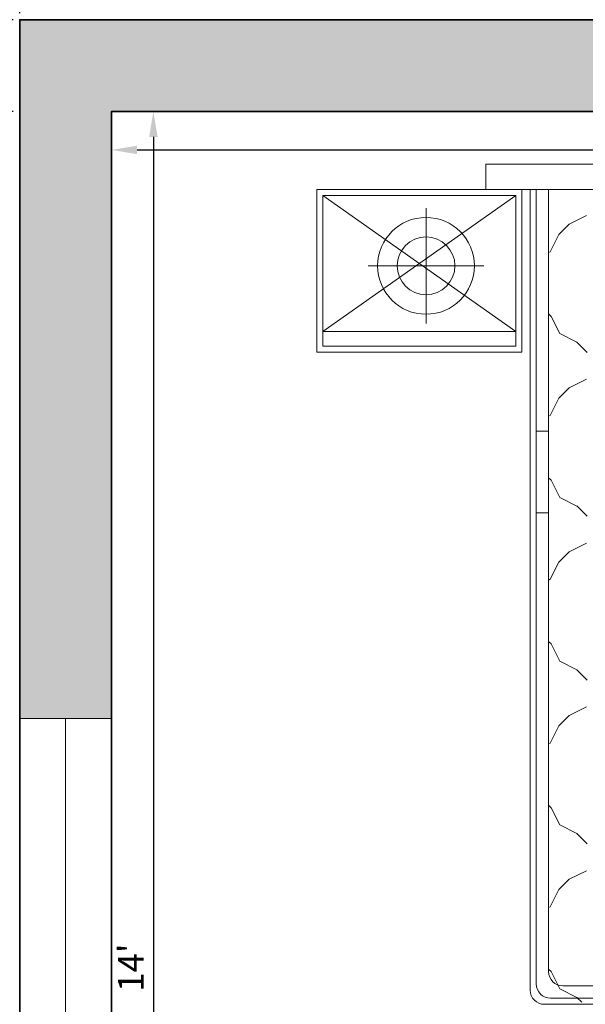
# Model space of a CAD drawing. Units: inches. Extents: x 2901 to 5923, y 918 to 2827.
# Tile 5 of 16: x 4430 to 4486, y 1534 to 1630. Entities that reach past the tile are written whole.
import ezdxf

# ---------------------------------------------------------------- set-up
doc = ezdxf.new("R2010")
doc.units = ezdxf.units.IN
for name, color, linetype, lineweight in [('A-ANNO-DIMS', 2, 'Continuous', 18), ('A-GLAZ', 4, 'Continuous', 18), ('A-WALL-PATT', 7, 'Continuous', 13), ('furniture', 160, 'Continuous', 18), ('walls', 7, 'Continuous', 35)]:
    doc.layers.add(name, color=color, linetype=linetype, lineweight=lineweight)
doc.styles.get("Standard").update_dxf_attribs({"font": 'arial.ttf'})
doc.dimstyles.new('Copy of ISO-25', dxfattribs={"dimtxt": 2.5, "dimasz": 2.5, "dimexe": 1.25, "dimexo": 0.625, "dimtad": 1, "dimdec": 1, "dimlunit": 4, "dimtxsty": 'Standard', "dimcen": 2.5, "dimadec": 0, "dimazin": 0, "dimtfac": 1, "dimtdec": 1, "dimtmove": 0, "dimatfit": 3, "dimfxl": 1, "dimarcsym": 0})

# ---------------------------------------------------------------- blocks, each defined once
blk = doc.blocks.new('A$C029D5C69')
for p, q in [((0.4164, 2.0693), (0.4164, 2.0066)), ((2.2315, 2.0693), (0.4164, 2.0693)), ((0, 1.606), (0, 2.0066)), ((0, 2.0066), (0.505, 2.0066)), ((0.0151, 1.6211), (0.0151, 1.9915)), ((0.0151, 1.9915), (0.4899, 1.9915)), ((0.4164, 2.0066), (2.2315, 2.0066)), ((0.4899, 1.9915), (0.4899, 1.6211)), ((0.505, 2.0066), (0.505, 1.606)), ((0.5252, 0.0351), (0.5252, 2.0066)), ((0.5403, 0.0502), (0.5403, 2.0066)), ((0.5706, 0.0805), (0.5706, 2.0066)), ((0.2689, 1.9609), (0.2689, 1.6764)), ((0.6634, 1.9425), (0.621, 1.9213)), ((0.6634, 1.9425), (0.621, 1.9213)), ((0.621, 1.9213), (0.5955, 1.8958)), ((0.5955, 1.8958), (0.5743, 1.8534)), ((0.5743, 1.8534), (0.5706, 1.8515)), ((0.5743, 1.8534), (0.5706, 1.8515)), ((0.1267, 1.8186), (0.4111, 1.8186)), ((0.5766, 1.6941), (0.5706, 1.7002)), ((0.5978, 1.6517), (0.5766, 1.6941)), ((0.6402, 1.6305), (0.5978, 1.6517)), ((0.6402, 1.6305), (0.5978, 1.6517)), ((0.6657, 1.605), (0.6402, 1.6305)), ((0.505, 1.606), (0, 1.606)), ((0.4899, 1.6211), (0.0151, 1.6211)), ((0.6634, 1.5391), (0.621, 1.5179)), ((0.6634, 1.5391), (0.621, 1.5179)), ((0.621, 1.5179), (0.5955, 1.4924)), ((0.5955, 1.4925), (0.5743, 1.4501)), ((0.5743, 1.45), (0.5706, 1.4481)), ((0.5743, 1.45), (0.5706, 1.4481)), ((0.5403, 1.4117), (0.5706, 1.4117)), ((0.5766, 1.2908), (0.5706, 1.2968)), ((0.5978, 1.2484), (0.5766, 1.2908)), ((0.6402, 1.2271), (0.5978, 1.2483)), ((0.6402, 1.2271), (0.5978, 1.2483)), ((0.6657, 1.2017), (0.6402, 1.2272)), ((0.5403, 1.21), (0.5706, 1.21)), ((0.6634, 1.1358), (0.621, 1.1146)), ((0.6634, 1.1358), (0.621, 1.1146)), ((0.621, 1.1146), (0.5955, 1.0891)), ((0.5955, 1.0891), (0.5743, 1.0467)), ((0.5743, 1.0467), (0.5706, 1.0448)), ((0.5743, 1.0467), (0.5706, 1.0448)), ((0.5766, 0.8874), (0.5706, 0.8935)), ((0.5978, 0.845), (0.5766, 0.8874)), ((0.6402, 0.8238), (0.5978, 0.845)), ((0.6402, 0.8238), (0.5978, 0.845)), ((0.6657, 0.7983), (0.6402, 0.8238)), ((0.6634, 0.7324), (0.621, 0.7112)), ((0.6634, 0.7324), (0.621, 0.7112)), ((0.621, 0.7113), (0.5955, 0.6858)), ((0.5955, 0.6858), (0.5743, 0.6434)), ((0.5743, 0.6433), (0.5706, 0.6414)), ((0.5743, 0.6433), (0.5706, 0.6414)), ((0.5766, 0.4841), (0.5706, 0.4901)), ((0.5978, 0.4417), (0.5766, 0.4841)), ((0.6402, 0.4205), (0.5978, 0.4417)), ((0.6402, 0.4205), (0.5978, 0.4417)), ((0.6657, 0.395), (0.6402, 0.4205)), ((0.6634, 0.3291), (0.621, 0.3079)), ((0.6634, 0.3291), (0.621, 0.3079)), ((0.621, 0.3079), (0.5955, 0.2824)), ((0.5955, 0.2824), (0.5743, 0.24)), ((0.5743, 0.24), (0.5706, 0.2381)), ((0.5743, 0.24), (0.5706, 0.2381)), ((0.5766, 0.0807), (0.5706, 0.0868)), ((0.5978, 0.0384), (0.5766, 0.0808)), ((0.6402, 0.0171), (0.5978, 0.0383)), ((0.6402, 0.0171), (0.5978, 0.0383)), ((2.0309, 0.0454), (0.6056, 0.0454)), ((2.0763, 0), (0.5603, 0)), ((2.0612, 0.0151), (0.5754, 0.0151)), ((0.6523, 0.005), (0.6402, 0.0171))]:
    blk.add_line(p, q)
at = {"ltscale": 0.005}
for p, q in [((0.4899, 1.6568), (0.0151, 1.9915)), ((0.0151, 1.6568), (0.4899, 1.9915)), ((0.0151, 1.6568), (0.4899, 1.6568))]:
    blk.add_line(p, q, dxfattribs=at)
for radius in [0.1191, 0.0711]:
    blk.add_circle((0.2689, 1.8186), radius)
for centre in [(0.6056, 0.0805), (0.5754, 0.0502), (0.5603, 0.0351)]:
    blk.add_arc(centre, 0.0351, 180, 270)
blk = doc.blocks.new('A$C0D3A6DFA')
blk.add_blockref('A$C029D5C69', (0, 0))
blk = doc.blocks.new('*D26')
at = {"layer": 'A-ANNO-DIMS', "color": 0, "lineweight": -2, "transparency": 16777216}
for p, q in [((4425.952, 1632.897), (4425.952, 1639.52)), ((4429.443, 1630.397), (4424.702, 1630.397)), ((4429.443, 1630.397), (4424.702, 1630.397)), ((4425.952, 1627.897), (4425.952, 1625.397))]:
    blk.add_line(p, q, dxfattribs=at)
at = {"layer": 'A-ANNO-DIMS', "color": 0, "transparency": 16777216}
for points in [[(4425.535, 1632.897), (4426.368, 1632.897), (4425.952, 1630.397)], [(4425.535, 1627.897), (4426.368, 1627.897), (4425.952, 1630.397)]]:
    blk.add_solid(points, dxfattribs=at)
at = {"layer": 'Defpoints', "color": 0, "transparency": 16777216}
for p in [(4425.952, 1630.397), (4430.068, 1630.397), (4430.068, 1630.397)]:
    blk.add_point(p, dxfattribs=at)
at = {"layer": 'A-ANNO-DIMS', "color": 0, "transparency": 16777216, "insert": (4424.05, 1637.458), "char_height": 2.5, "attachment_point": 5, "rotation": 90}
blk.add_mtext('0"', dxfattribs=at)
blk = doc.blocks.new('*D27')
at = {"layer": 'A-ANNO-DIMS', "color": 0, "lineweight": -2, "transparency": 16777216}
for p, q in [((4429.443, 1621.397), (4424.639, 1621.397)), ((4425.889, 1618.897), (4425.889, 1248.897)), ((4429.443, 1246.397), (4424.639, 1246.397))]:
    blk.add_line(p, q, dxfattribs=at)
at = {"layer": 'A-ANNO-DIMS', "color": 0, "transparency": 16777216}
for points in [[(4425.473, 1618.897), (4426.306, 1618.897), (4425.889, 1621.397)], [(4425.473, 1248.897), (4426.306, 1248.897), (4425.889, 1246.397)]]:
    blk.add_solid(points, dxfattribs=at)
at = {"layer": 'Defpoints', "color": 0, "transparency": 16777216}
for p in [(4430.068, 1621.397), (4425.889, 1246.397), (4430.068, 1246.397)]:
    blk.add_point(p, dxfattribs=at)
at = {"layer": 'A-ANNO-DIMS', "color": 0, "transparency": 16777216, "insert": (4423.987, 1433.897), "char_height": 2.5, "attachment_point": 5, "rotation": 90}
blk.add_mtext('31\'-3"', dxfattribs=at)
blk = doc.blocks.new('*D36')
at = {"layer": 'A-ANNO-DIMS', "color": 0, "lineweight": -2, "transparency": 16777216}
for p, q in [((4430.068, 1631.022), (4430.068, 1640.2)), ((4892.068, 1631.022), (4892.068, 1640.2)), ((4432.568, 1638.95), (4889.568, 1638.95))]:
    blk.add_line(p, q, dxfattribs=at)
at = {"layer": 'A-ANNO-DIMS', "color": 0, "transparency": 16777216}
for points in [[(4432.568, 1639.367), (4432.568, 1638.533), (4430.068, 1638.95)], [(4889.568, 1639.367), (4889.568, 1638.533), (4892.068, 1638.95)]]:
    blk.add_solid(points, dxfattribs=at)
at = {"layer": 'Defpoints', "color": 0, "transparency": 16777216}
for p in [(4892.068, 1638.95), (4430.068, 1630.397), (4892.068, 1630.397)]:
    blk.add_point(p, dxfattribs=at)
at = {"layer": 'A-ANNO-DIMS', "color": 0, "transparency": 16777216, "insert": (4661.068, 1640.852), "char_height": 2.5, "attachment_point": 5}
blk.add_mtext('38\'-6"', dxfattribs=at)
blk = doc.blocks.new('*D39')
at = {"layer": 'A-ANNO-DIMS', "color": 0, "lineweight": -2, "transparency": 16777216}
for p, q in [((4439.068, 1620.772), (4439.068, 1616.368)), ((4583.068, 1620.772), (4583.068, 1616.368)), ((4441.568, 1617.618), (4580.568, 1617.618))]:
    blk.add_line(p, q, dxfattribs=at)
at = {"layer": 'A-ANNO-DIMS', "color": 0, "transparency": 16777216}
for points in [[(4441.568, 1618.034), (4441.568, 1617.201), (4439.068, 1617.618)], [(4580.568, 1618.034), (4580.568, 1617.201), (4583.068, 1617.618)]]:
    blk.add_solid(points, dxfattribs=at)
at = {"layer": 'Defpoints', "color": 0, "transparency": 16777216}
for p in [(4439.068, 1621.397), (4583.068, 1621.397), (4583.068, 1617.618)]:
    blk.add_point(p, dxfattribs=at)
at = {"layer": 'A-ANNO-DIMS', "color": 0, "transparency": 16777216, "insert": (4511.068, 1619.498), "char_height": 2.5, "attachment_point": 5}
blk.add_mtext("12'", dxfattribs=at)
blk = doc.blocks.new('*D40')
at = {"layer": 'A-ANNO-DIMS', "color": 0, "lineweight": -2, "transparency": 16777216}
for p, q in [((4439.693, 1621.397), (4444.423, 1621.397)), ((4443.173, 1618.897), (4443.173, 1455.897)), ((4439.693, 1453.397), (4444.423, 1453.397))]:
    blk.add_line(p, q, dxfattribs=at)
at = {"layer": 'A-ANNO-DIMS', "color": 0, "transparency": 16777216}
for points in [[(4442.756, 1618.897), (4443.59, 1618.897), (4443.173, 1621.397)], [(4442.756, 1455.897), (4443.59, 1455.897), (4443.173, 1453.397)]]:
    blk.add_solid(points, dxfattribs=at)
at = {"layer": 'Defpoints', "color": 0, "transparency": 16777216}
for p in [(4439.068, 1621.397), (4439.068, 1453.397), (4443.173, 1453.397)]:
    blk.add_point(p, dxfattribs=at)
at = {"layer": 'A-ANNO-DIMS', "color": 0, "transparency": 16777216, "insert": (4441.293, 1537.397), "char_height": 2.5, "attachment_point": 5, "rotation": 90}
blk.add_mtext("14'", dxfattribs=at)

msp = doc.modelspace()

# ---------------------------------------------------------------- hatches: boundary and pattern name
at = {"layer": 'A-WALL-PATT'}
h = msp.add_hatch(color=256, dxfattribs=at)
h.dxf.hatch_style = 1
h.paths.add_polyline_path([(4439.068, 1447.397), (4583.068, 1447.397), (4583.068, 1340.397), (4589.068, 1340.397), (4589.068, 1453.397), (4589.068, 1455.386), (4583.068, 1455.386), (4583.068, 1453.397), (4439.068, 1453.397), (4439.068, 1501.839), (4430.068, 1501.839), (4430.068, 1399.397), (4439.068, 1399.397)])
h.paths.add_polyline_path([(4439.068, 1621.397), (4487.068, 1621.397), (4487.068, 1630.397), (4430.068, 1630.397), (4430.068, 1561.839), (4439.068, 1561.839)])
h.paths.add_polyline_path([(4630.605, 1630.397), (4535.068, 1630.397), (4535.068, 1621.397), (4583.068, 1621.397), (4583.068, 1495.397), (4589.068, 1495.397), (4637.068, 1495.397), (4637.068, 1501.397), (4589.068, 1501.397), (4589.068, 1621.397), (4630.605, 1621.397)])
h.paths.add_polyline_path([(4892.068, 1630.397), (4690.605, 1630.397), (4690.605, 1621.397), (4733.068, 1621.397), (4733.068, 1564.397), (4739.068, 1564.397), (4739.068, 1621.397), (4883.068, 1621.397), (4883.068, 1528.397), (4739.068, 1528.397), (4733.068, 1528.397), (4733.068, 1501.397), (4685.068, 1501.397), (4685.068, 1495.397), (4739.068, 1495.397), (4739.068, 1519.397), (4787.068, 1519.397), (4787.068, 1423.397), (4739.068, 1423.397), (4739.068, 1456.668), (4733.068, 1456.668), (4733.068, 1340.397), (4739.068, 1340.397), (4739.068, 1417.397), (4787.068, 1417.397), (4793.068, 1417.397), (4793.068, 1423.397), (4793.068, 1519.397), (4883.068, 1519.397), (4883.068, 1482.87), (4892.068, 1482.87)])
h.paths.add_polyline_path([(4892.068, 1458.87), (4883.068, 1458.87), (4883.068, 1423.397), (4823.068, 1423.397), (4823.068, 1417.397), (4883.068, 1417.397), (4883.068, 1363.306), (4892.068, 1363.306)], flags=17)
h.paths.add_polyline_path([(4892.068, 1303.306), (4883.068, 1303.306), (4883.068, 1255.397), (4739.068, 1255.397), (4739.068, 1304.397), (4733.068, 1304.397), (4733.068, 1303.397), (4733.068, 1297.397), (4733.068, 1255.397), (4733.068, 1248.397), (4811.068, 1248.397), (4811.068, 1212.161), (4820.068, 1212.161), (4820.068, 1248.397), (4892.068, 1248.397)])
h.paths.add_polyline_path([(4820.068, 1182.161), (4811.068, 1182.161), (4811.068, 1152.397), (4685.068, 1152.397), (4685.068, 1147.029), (4685.068, 1143.397), (4733.068, 1143.397), (4811.068, 1143.397), (4814.068, 1143.397), (4820.068, 1143.397)])
h.paths.add_polyline_path([(4637.068, 1152.397), (4589.068, 1152.397), (4589.068, 1153.397), (4583.863, 1153.397), (4583.068, 1153.397), (4583.068, 1152.397), (4511.068, 1152.397), (4511.068, 1182.161), (4502.068, 1182.161), (4502.068, 1143.397), (4568.068, 1143.397), (4583.068, 1143.397), (4583.068, 1023.397), (4739.068, 1023.397), (4739.068, 1143.397), (4733.068, 1143.397), (4733.068, 1029.397), (4589.068, 1029.397), (4589.068, 1143.397), (4637.068, 1143.397), (4637.068, 1146.969)])
h.paths.add_polyline_path([(4511.068, 1246.397), (4583.068, 1246.397), (4583.068, 1188.397), (4589.068, 1188.397), (4589.068, 1246.397), (4589.068, 1248.397), (4589.068, 1255.397), (4589.068, 1297.397), (4697.068, 1297.397), (4697.068, 1303.397), (4589.068, 1303.397), (4589.068, 1304.397), (4583.068, 1304.397), (4583.068, 1255.397), (4439.068, 1255.397), (4439.068, 1261.397), (4439.068, 1351.397), (4430.068, 1351.397), (4430.068, 1252.397), (4430.068, 1246.397), (4439.068, 1246.397), (4487.068, 1246.397), (4502.068, 1246.397), (4502.068, 1212.161), (4511.068, 1212.161)])

# ---------------------------------------------------------------- linework, layer by layer
at = {"layer": 'A-GLAZ'}
for p, q in [((4439.068, 1561.839), (4430.068, 1561.839)), ((4430.068, 1561.839), (4430.068, 1501.839)), ((4434.568, 1561.839), (4434.568, 1501.839))]:
    msp.add_line(p, q, dxfattribs=at)
at = {"layer": 'walls'}
for q in [(4583.068, 1621.397), (4439.068, 1561.839)]:
    msp.add_line((4439.068, 1621.397), q, dxfattribs=at)
for points in [[(4892.068, 1630.397), (4430.068, 1630.397), (4430.068, 1252.397)], [(4583.068, 1621.397), (4439.068, 1621.397), (4439.068, 1453.397)]]:
    msp.add_lwpolyline(points, dxfattribs=at)

# ---------------------------------------------------------------- block references
at = {"layer": 'furniture', "xscale": 39.84014367312396, "yscale": 39.84014367312396, "zscale": 39.84014367312396}
msp.add_blockref('A$C0D3A6DFA', (4459.192, 1533.796), dxfattribs=at)

# ---------------------------------------------------------------- dimensions: what is measured, and where the dimension line sits
at = {"layer": 'A-ANNO-DIMS'}
for base, p1, p2, picture, middle in [((4892.068, 1638.95), (4430.068, 1630.397), (4892.068, 1630.397), '*D36', (4661.068, 1640.852)), ((4583.068, 1617.618), (4439.068, 1621.397), (4583.068, 1621.397), '*D39', (4511.068, 1619.498))]:
    dim = msp.add_linear_dim(base=base, p1=p1, p2=p2, dimstyle='Copy of ISO-25', override={"dimclrd": 0, "dimclre": 0, "dimclrt": 0}, dxfattribs=at)
    dim.commit()
    dim.dimension.update_dxf_attribs({"geometry": picture, "text_midpoint": middle})
for base, p1, p2, picture, middle in [((4425.951791153, 1630.396623547), (4430.068422296, 1630.396623547), (4430.068422296, 1630.396623547), '*D26', (4424.050358683, 1637.458356153)), ((4425.889, 1246.397), (4430.068, 1621.397), (4430.068, 1246.397), '*D27', (4423.987, 1433.897)), ((4443.173, 1453.397), (4439.068, 1621.397), (4439.068, 1453.397), '*D40', (4441.293, 1537.397))]:
    dim = msp.add_linear_dim(base=base, p1=p1, p2=p2, angle=90, dimstyle='Copy of ISO-25', override={"dimclrd": 0, "dimclre": 0, "dimclrt": 0}, dxfattribs=at)
    dim.commit()
    dim.dimension.update_dxf_attribs({"geometry": picture, "text_midpoint": middle})

doc.saveas('drawing.dxf')
